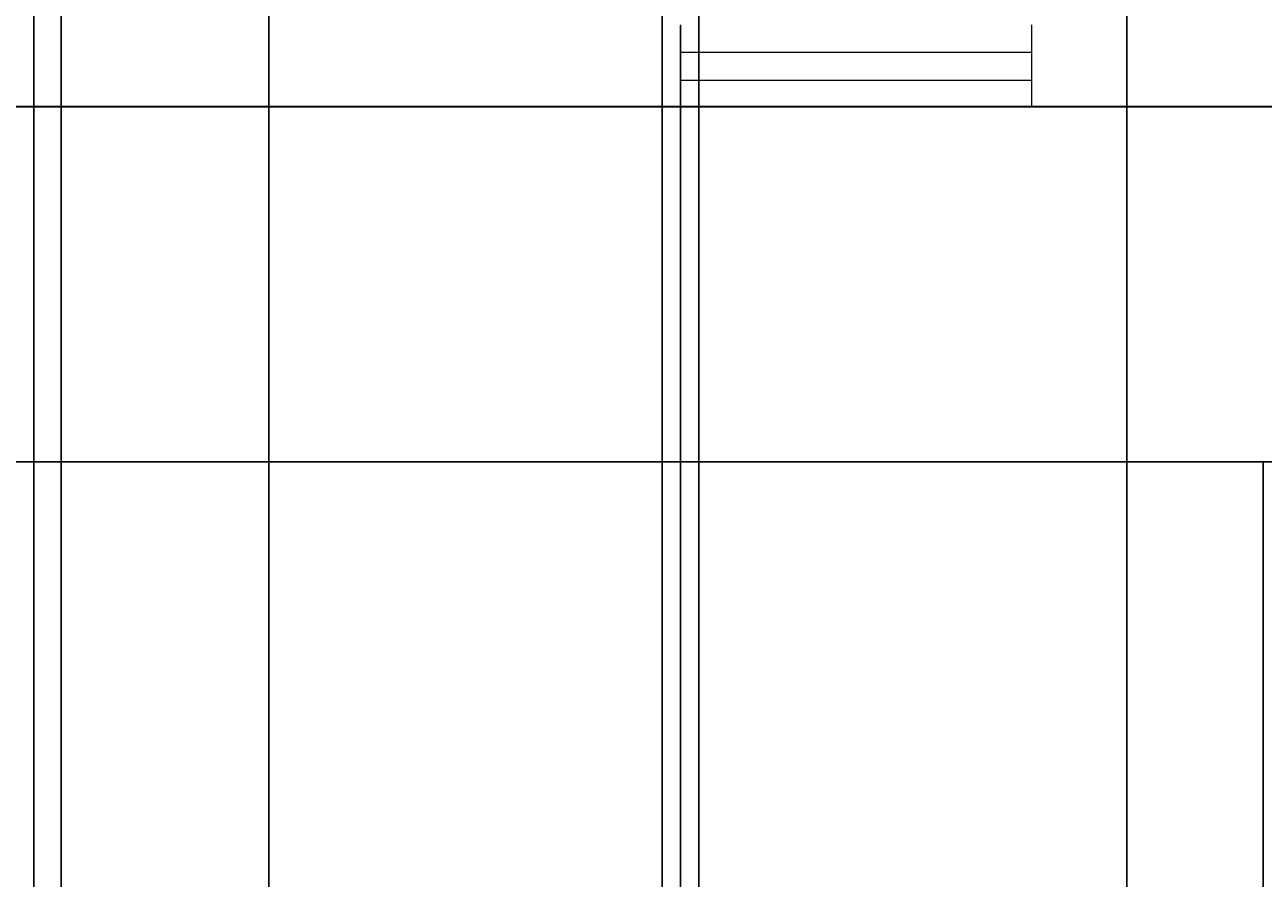
# Model space of a CAD drawing. Units: inches. Extents: x 867 to 1667, y -234 to 788.
# Tile 7 of 42: x 1076 to 1212, y -102 to -8. Entities that reach past the tile are written whole.
import ezdxf

# ---------------------------------------------------------------- set-up
doc = ezdxf.new("R2010")
doc.units = ezdxf.units.IN
doc.header["$MEASUREMENT"] = 0
for name, color, linetype, lineweight in [('A-ANNO-DIMS', 2, 'Continuous', 18), ('A-FLOR-OTLN', 7, 'Continuous', 25), ('A-Glaz', 92, 'Continuous', 18), ('A-Wall', 7, 'Continuous', 35)]:
    doc.layers.add(name, color=color, linetype=linetype, lineweight=lineweight)
doc.styles.get("Standard").update_dxf_attribs({"font": 'arial.ttf'})
doc.dimstyles.get("Standard").update_dxf_attribs({"dimtxt": 0.6875, "dimasz": 0.18, "dimexe": 0.18, "dimexo": 0.0625, "dimgap": 0.09, "dimtad": 0, "dimdec": 4, "dimzin": 0, "dimdsep": 46, "dimlunit": 4, "dimtxsty": 'Standard', "dimcen": 0.09, "dimadec": 0, "dimazin": 0, "dimtfac": 1, "dimtdec": 4, "dimtofl": 0, "dimtmove": 0, "dimatfit": 3, "dimfxl": 1, "dimtolj": 1, "dimtzin": 0, "dimarcsym": 0})

# ---------------------------------------------------------------- blocks, each defined once
blk = doc.blocks.new('WIN-38_58IN')
for p, q in [((0, 9), (0, 0)), ((38.58, 0), (38.58, 9)), ((0, 6), (38.58, 6)), ((0, 2.92), (38.58, 2.92)), ((0, 0), (38.58, 0))]:
    blk.add_line(p, q)
blk = doc.blocks.new('*D27')
at = {"layer": 'A-ANNO-DIMS', "color": 0, "lineweight": -2, "transparency": 16777216}
for p, q in [((1070.89, -55.97), (1070.89, -233.54)), ((1525.26, -186.47), (1525.26, -233.54)), ((1071.07, -233.36), (1296.81, -233.36)), ((1525.08, -233.36), (1299.34, -233.36))]:
    blk.add_line(p, q, dxfattribs=at)
at = {"layer": 'A-ANNO-DIMS', "color": 0, "transparency": 16777216}
for points in [[(1071.07, -233.33), (1071.07, -233.39), (1070.89, -233.36)], [(1525.08, -233.33), (1525.08, -233.39), (1525.26, -233.36)]]:
    blk.add_solid(points, dxfattribs=at)
at = {"layer": 'Defpoints', "color": 0, "transparency": 16777216}
for p in [(1070.89, -55.91), (1525.26, -186.41), (1525.26, -233.36)]:
    blk.add_point(p, dxfattribs=at)
at = {"layer": 'A-ANNO-DIMS', "color": 0, "transparency": 16777216, "insert": (1298.08, -233.36), "char_height": 0.688, "attachment_point": 5}
blk.add_mtext('\\A1;454.4', dxfattribs=at)
blk = doc.blocks.new('*D29')
at = {"layer": 'A-ANNO-DIMS', "color": 0, "lineweight": -2, "transparency": 16777216}
for p, q in [((1076.89, 623.55), (1076.89, -233.54)), ((1102.67, 623.55), (1102.67, -233.54)), ((1077.07, -233.36), (1088.52, -233.36)), ((1102.49, -233.36), (1091.03, -233.36))]:
    blk.add_line(p, q, dxfattribs=at)
at = {"layer": 'A-ANNO-DIMS', "color": 0, "transparency": 16777216}
for points in [[(1077.07, -233.33), (1077.07, -233.39), (1076.89, -233.36)], [(1102.49, -233.33), (1102.49, -233.39), (1102.67, -233.36)]]:
    blk.add_solid(points, dxfattribs=at)
at = {"layer": 'Defpoints', "color": 0, "transparency": 16777216}
for p in [(1076.89, 623.62), (1102.67, 623.62), (1102.67, -233.36)]:
    blk.add_point(p, dxfattribs=at)
at = {"layer": 'A-ANNO-DIMS', "color": 0, "transparency": 16777216, "insert": (1089.78, -233.36), "char_height": 0.688, "attachment_point": 5}
blk.add_mtext('\\A1;25.78', dxfattribs=at)
blk = doc.blocks.new('*D37')
at = {"layer": 'A-ANNO-DIMS', "color": 0, "lineweight": -2, "transparency": 16777216}
for p, q in [((1049.89, 257.55), (1049.89, -233.54)), ((1196.89, 257.55), (1196.89, -233.54)), ((1050.07, -233.36), (1122.57, -233.36)), ((1196.71, -233.36), (1124.2, -233.36))]:
    blk.add_line(p, q, dxfattribs=at)
at = {"layer": 'A-ANNO-DIMS', "color": 0, "transparency": 16777216}
for points in [[(1050.07, -233.33), (1050.07, -233.39), (1049.89, -233.36)], [(1196.71, -233.33), (1196.71, -233.39), (1196.89, -233.36)]]:
    blk.add_solid(points, dxfattribs=at)
at = {"layer": 'Defpoints', "color": 0, "transparency": 16777216}
for p in [(1049.89, 257.62), (1196.89, 257.62), (1196.89, -233.36)]:
    blk.add_point(p, dxfattribs=at)
at = {"layer": 'A-ANNO-DIMS', "color": 0, "transparency": 16777216, "insert": (1123.39, -233.36), "char_height": 0.688, "attachment_point": 5}
blk.add_mtext('\\A1;147', dxfattribs=at)
blk = doc.blocks.new('*D42')
at = {"layer": 'A-ANNO-DIMS', "color": 0, "lineweight": -2, "transparency": 16777216}
for p, q in [((1079.89, 136.05), (1079.89, -233.54)), ((1145.89, 136.05), (1145.89, -233.54)), ((1080.07, -233.36), (1112.3, -233.36)), ((1145.71, -233.36), (1113.47, -233.36))]:
    blk.add_line(p, q, dxfattribs=at)
at = {"layer": 'A-ANNO-DIMS', "color": 0, "transparency": 16777216}
for points in [[(1080.07, -233.33), (1080.07, -233.39), (1079.89, -233.36)], [(1145.71, -233.33), (1145.71, -233.39), (1145.89, -233.36)]]:
    blk.add_solid(points, dxfattribs=at)
at = {"layer": 'Defpoints', "color": 0, "transparency": 16777216}
for p in [(1079.89, 136.12), (1145.89, 136.12), (1145.89, -233.36)]:
    blk.add_point(p, dxfattribs=at)
at = {"layer": 'A-ANNO-DIMS', "color": 0, "transparency": 16777216, "insert": (1112.89, -233.36), "char_height": 0.688, "attachment_point": 5}
blk.add_mtext('\\A1;66', dxfattribs=at)
blk = doc.blocks.new('*D43')
at = {"layer": 'A-ANNO-DIMS', "color": 0, "lineweight": -2, "transparency": 16777216}
for p, q in [((1145.89, 136.05), (1145.89, -233.54)), ((1149.89, 136.05), (1149.89, -233.54)), ((1146.07, -233.36), (1147.56, -233.36)), ((1149.71, -233.36), (1148.21, -233.36))]:
    blk.add_line(p, q, dxfattribs=at)
at = {"layer": 'A-ANNO-DIMS', "color": 0, "transparency": 16777216}
for points in [[(1146.07, -233.33), (1146.07, -233.39), (1145.89, -233.36)], [(1149.71, -233.33), (1149.71, -233.39), (1149.89, -233.36)]]:
    blk.add_solid(points, dxfattribs=at)
at = {"layer": 'Defpoints', "color": 0, "transparency": 16777216}
for p in [(1145.89, 136.12), (1149.89, 136.12), (1149.89, -233.36)]:
    blk.add_point(p, dxfattribs=at)
at = {"layer": 'A-ANNO-DIMS', "color": 0, "transparency": 16777216, "insert": (1147.89, -233.36), "char_height": 0.688, "attachment_point": 5}
blk.add_mtext('\\A1;4', dxfattribs=at)
blk = doc.blocks.new('*D45')
at = {"layer": 'A-ANNO-DIMS', "color": 0, "lineweight": -2, "transparency": 16777216}
for p, q in [((1079.89, -7.95), (1079.89, -233.54)), ((1247.89, -7.95), (1247.89, -233.54)), ((1080.07, -233.36), (1163.07, -233.36)), ((1247.71, -233.36), (1164.7, -233.36))]:
    blk.add_line(p, q, dxfattribs=at)
at = {"layer": 'A-ANNO-DIMS', "color": 0, "transparency": 16777216}
for points in [[(1080.07, -233.33), (1080.07, -233.39), (1079.89, -233.36)], [(1247.71, -233.33), (1247.71, -233.39), (1247.89, -233.36)]]:
    blk.add_solid(points, dxfattribs=at)
at = {"layer": 'Defpoints', "color": 0, "transparency": 16777216}
for p in [(1079.89, -7.88), (1247.89, -7.88), (1247.89, -233.36)]:
    blk.add_point(p, dxfattribs=at)
at = {"layer": 'A-ANNO-DIMS', "color": 0, "transparency": 16777216, "insert": (1163.89, -233.36), "char_height": 0.688, "attachment_point": 5}
blk.add_mtext('\\A1;168', dxfattribs=at)
blk = doc.blocks.new('*D49')
at = {"layer": 'A-ANNO-DIMS', "color": 0, "lineweight": -2, "transparency": 16777216}
for p, q in [((1070.89, -55.97), (1070.89, -233.54)), ((1211.89, -55.97), (1211.89, -233.54)), ((1071.07, -233.36), (1140.64, -233.36)), ((1211.71, -233.36), (1142.14, -233.36))]:
    blk.add_line(p, q, dxfattribs=at)
at = {"layer": 'A-ANNO-DIMS', "color": 0, "transparency": 16777216}
for points in [[(1071.07, -233.33), (1071.07, -233.39), (1070.89, -233.36)], [(1211.71, -233.33), (1211.71, -233.39), (1211.89, -233.36)]]:
    blk.add_solid(points, dxfattribs=at)
at = {"layer": 'Defpoints', "color": 0, "transparency": 16777216}
for p in [(1070.89, -55.91), (1211.89, -55.91), (1211.89, -233.36)]:
    blk.add_point(p, dxfattribs=at)
at = {"layer": 'A-ANNO-DIMS', "color": 0, "transparency": 16777216, "insert": (1141.39, -233.36), "char_height": 0.688, "attachment_point": 5}
blk.add_mtext('\\A1;141', dxfattribs=at)
blk = doc.blocks.new('*D57')
at = {"layer": 'A-ANNO-DIMS', "color": 0, "lineweight": -2, "transparency": 16777216}
for p, q in [((1079.89, -7.95), (1079.89, -233.54)), ((1147.89, -7.95), (1147.89, -233.54)), ((1080.07, -233.36), (1113.3, -233.36)), ((1147.71, -233.36), (1114.47, -233.36))]:
    blk.add_line(p, q, dxfattribs=at)
at = {"layer": 'A-ANNO-DIMS', "color": 0, "transparency": 16777216}
for points in [[(1080.07, -233.33), (1080.07, -233.39), (1079.89, -233.36)], [(1147.71, -233.33), (1147.71, -233.39), (1147.89, -233.36)]]:
    blk.add_solid(points, dxfattribs=at)
at = {"layer": 'Defpoints', "color": 0, "transparency": 16777216}
for p in [(1079.89, -7.88), (1147.89, -7.88), (1147.89, -233.36)]:
    blk.add_point(p, dxfattribs=at)
at = {"layer": 'A-ANNO-DIMS', "color": 0, "transparency": 16777216, "insert": (1113.89, -233.36), "char_height": 0.688, "attachment_point": 5}
blk.add_mtext('\\A1;68', dxfattribs=at)

msp = doc.modelspace()

# ---------------------------------------------------------------- linework, layer by layer
at = {"layer": 'A-FLOR-OTLN'}
msp.add_line((1070.8866, -55.9081), (1283.8866, -55.9081), dxfattribs=at)
at = {"layer": 'A-Wall'}
msp.add_line((1283.8866, -16.883), (1070.8866, -16.883), dxfattribs=at)

# ---------------------------------------------------------------- block references
at = {"layer": 'A-Glaz'}
msp.add_blockref('WIN-38_58IN', (1147.8923, -16.883), dxfattribs=at)

# ---------------------------------------------------------------- dimensions: what is measured, and where the dimension line sits
at = {"layer": 'A-ANNO-DIMS'}
for base, p1, p2, override, picture, middle in [((1102.6661, -233.3581), (1076.8866, 623.617), (1102.6661, 623.617), {"dimdec": 2, "dimlfac": 1, "dimrnd": 0, "dimzin": 0, "dimdsep": 46, "dimlunit": 2}, '*D29', (1089.7763, -233.3581)), ((1196.8866, -233.3581), (1049.8866, 257.617), (1196.8866, 257.617), {"dimdec": 0, "dimlfac": 1, "dimrnd": 0, "dimzin": 0, "dimdsep": 46, "dimlunit": 2}, '*D37', (1123.3866, -233.3581)), ((1145.8866, -233.3581), (1079.8866, 136.117), (1145.8866, 136.117), {"dimdec": 0, "dimlfac": 1, "dimrnd": 0, "dimzin": 0, "dimdsep": 46, "dimlunit": 2}, '*D42', (1112.8866, -233.3581)), ((1149.8866, -233.3581), (1145.8866, 136.117), (1149.8866, 136.117), {"dimdec": 0, "dimlfac": 1, "dimrnd": 0, "dimzin": 0, "dimdsep": 46, "dimlunit": 2}, '*D43', (1147.8866, -233.3581)), ((1247.8866, -233.3581), (1079.8866, -7.883), (1247.8866, -7.883), {"dimdec": 0, "dimlfac": 1, "dimrnd": 0, "dimzin": 0, "dimdsep": 46, "dimlunit": 2}, '*D45', (1163.8866, -233.3581)), ((1147.8918, -233.3581), (1079.8866, -7.883), (1147.8918, -7.883), {"dimdec": 0, "dimlfac": 1, "dimrnd": 0, "dimzin": 0, "dimdsep": 46, "dimlunit": 2}, '*D57', (1113.8892, -233.3581)), ((1525.2648, -233.3581), (1070.8866, -55.9081), (1525.2648, -186.4081), {"dimdec": 1, "dimlfac": 1, "dimrnd": 0, "dimzin": 0, "dimdsep": 46, "dimlunit": 2}, '*D27', (1298.0757, -233.3581)), ((1211.8866, -233.3581), (1070.8866, -55.9081), (1211.8866, -55.9081), {"dimdec": 0, "dimlfac": 1, "dimrnd": 0, "dimzin": 0, "dimdsep": 46, "dimlunit": 2}, '*D49', (1141.3866, -233.3581))]:
    dim = msp.add_linear_dim(base=base, p1=p1, p2=p2, dimstyle='Standard', override=override, dxfattribs=at)
    dim.commit()
    dim.dimension.update_dxf_attribs({"geometry": picture, "text_midpoint": middle})

doc.saveas('drawing.dxf')
